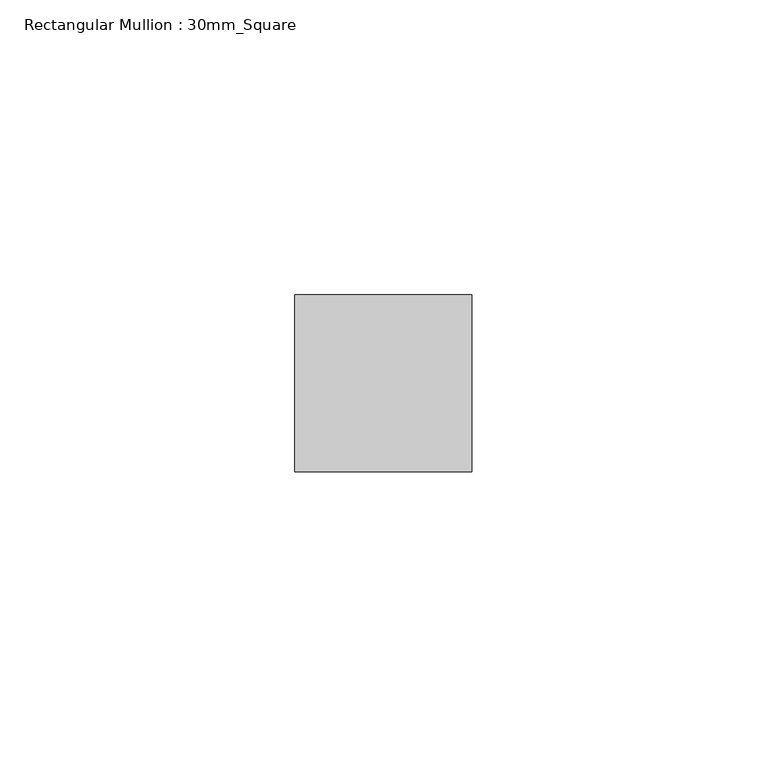
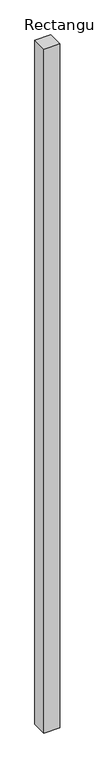
"""IFC4 building model written with IfcOpenShell, lengths in millimetres: member geometry, Rectangular Mullion : 30mm_Square."""

from ifc_helpers import new_model, si_unit, frame, origin, place, context, project, spatial, polyline, outline, extrude, source, transform, mapped, element, save


def rectangular_mullion_30mm_square_a54bfe06(model_context):
    return source(origin(), model_context, "Body", "SweptSolid", [
        extrude(outline(polyline([(0.0, 15.0), (0.0, -15.0), (-30.0, -15.0), (-30.0, 15.0), (0.0, 15.0)])), frame((0.0, 0.0, -1381.1782296), z_axis=(0.0, 0.0, 1.0), x_axis=(1.0, 0.0, 0.0)), (0.0, 0.0, 1.0), 1381.1782296),
    ])


if __name__ == "__main__":
    model = new_model("IFC4")
    model_context = context("Model", 3, world=origin())
    ifc_project = project(units=[si_unit("LENGTHUNIT", "METRE", prefix="MILLI")], contexts=[model_context])
    site = spatial("IfcSite", under=ifc_project)
    building = spatial("IfcBuilding", under=site)
    placement = place(None, origin())
    rectangular_mullion_30mm_square_shape = rectangular_mullion_30mm_square_a54bfe06(model_context)
    element("IfcMember", 1, ObjectType="Rectangular Mullion : 30mm_Square", at=placement, inside=building, context=model_context, shape_type="MappedRepresentation", body=[
        mapped(rectangular_mullion_30mm_square_shape, transform((0.0, 0.0, 0.0), x_axis=(1.0, 0.0, 0.0), y_axis=(0.0, 1.0, 0.0), z_axis=(0.0, 0.0, 1.0))),
    ])
    save(model, "model.ifc")

# Revit data of these elements
# Type "Rectangular Mullion : 30mm_Square"
#   Keynote = "H11"
#   built-in parameter 1007304 = 0.0984252 (stored number, unit not read)
#   built-in parameter 1007301 = 0.0492126 (stored number, unit not read)
#   built-in parameter 1007300 = 0.0492126 (stored number, unit not read)
# Element 1 (IfcMember, "Rectangular Mullion : 30mm_Square")
#   Materials on its faces: "Aluminium"
# Materials
#   "Aluminium": class "Metal", colour RGB 247 247 247, transparency 0, Description = "Aluminium 6061", Cost = 0
